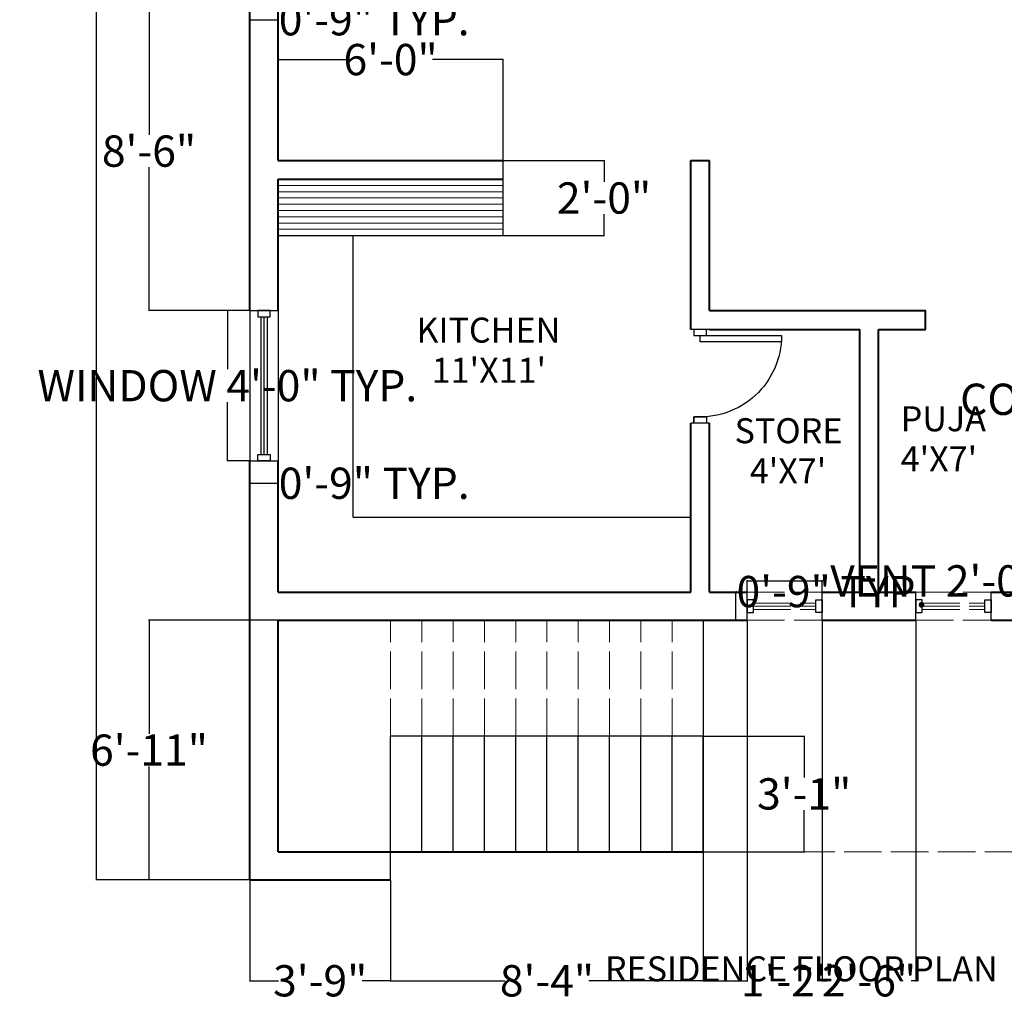
# Model space of a CAD drawing. Units: inches. Extents: x -413 to 212, y 1694 to 2633.
# Tile 2 of 5: x -413 to -98, y 1966 to 2279. Entities that reach past the tile are written whole.
import ezdxf

# ---------------------------------------------------------------- set-up
doc = ezdxf.new("R2010")
doc.units = ezdxf.units.IN
doc.header["$MEASUREMENT"] = 0
doc.linetypes.add('ACAD_ISO02W100', pattern=[15, 12, -3])
for name, color, linetype, lineweight in [('A-ANNO-DIMS', 5, 'Continuous', 18), ('A-ANNO-TEXT', 251, 'Continuous', 35), ('A-AREA-IDEN', 251, 'Continuous', 25), ('A-FLOR-FIXT', 1, 'Continuous', 25), ('A-FLOR-FIXT-PATT', 1, 'Continuous', 13), ('A-FLOR-OVHD', 20, 'ACAD_ISO02W100', 18), ('A-FLOR-STRS-OVHD', 3, 'ACAD_ISO02W100', 18), ('A-GLAZ-OVHD', 2, 'ACAD_ISO02W100', 18), ('A-GLAZ-VENT', 2, 'Continuous', 25), ('door', 4, 'Continuous', 25), ('stair case', 3, 'Continuous', 25), ('wall', 20, 'Continuous', 40), ('window', 6, 'Continuous', 25)]:
    doc.layers.add(name, color=color, linetype=linetype, lineweight=lineweight)
doc.styles.get("Standard").update_dxf_attribs({"font": 'arial.ttf'})
doc.dimstyles.get("Standard").update_dxf_attribs({"dimtxt": 10, "dimasz": 0.18, "dimexe": 0.18, "dimexo": 0.0625, "dimgap": 0.09, "dimtad": 0, "dimtih": 1, "dimtoh": 1, "dimdec": 1, "dimzin": 0, "dimdsep": 46, "dimlunit": 3, "dimtxsty": 'Standard', "dimblk": 'ARCHTICK', "dimcen": 0.09, "dimadec": 0, "dimazin": 0, "dimtfac": 1, "dimtdec": 1, "dimtofl": 0, "dimtmove": 0, "dimatfit": 3, "dimfxl": 1, "dimtolj": 1, "dimtzin": 0, "dimarcsym": 0})

# ---------------------------------------------------------------- blocks, each defined once
blk = doc.blocks.new('_ArchTick')
at = {"color": 0, "linetype": 'ByBlock', "const_width": 0.15}
blk.add_lwpolyline([(-0.5, -0.5), (0.5, 0.5)], dxfattribs=at)
blk = doc.blocks.new('*D2')
at = {"layer": 'A-ANNO-DIMS', "color": 0, "lineweight": -2, "transparency": 16777216}
for p, q in [((-339.04, 2585.48), (-388.23, 2585.48)), ((-388.05, 2585.48), (-388.05, 2300.18)), ((-388.05, 2004.48), (-388.05, 2289.79)), ((-339.04, 2004.48), (-388.23, 2004.48))]:
    blk.add_line(p, q, dxfattribs=at)
at = {"layer": 'Defpoints', "color": 0, "transparency": 16777216}
for p in [(-388.05, 2585.48), (-338.98, 2585.48), (-338.98, 2004.48)]:
    blk.add_point(p, dxfattribs=at)
at = {"layer": 'A-ANNO-DIMS', "color": 0, "lineweight": -2, "transparency": 16777216, "xscale": 0.18, "yscale": 0.18, "zscale": 0.18}
for p, rotation in [((-388.05, 2585.48), 90), ((-388.05, 2004.48), 270)]:
    blk.add_blockref('_ArchTick', p, dxfattribs=dict(at, rotation=rotation))
at = {"layer": 'A-ANNO-DIMS', "color": 0, "transparency": 16777216, "insert": (-388.05, 2294.98), "char_height": 10, "attachment_point": 5}
blk.add_mtext('\\A1;48\'-5.0"', dxfattribs=at)
blk = doc.blocks.new('WINDOW-48IN')
for p, q in [((0, 0), (0, 9)), ((0, 9), (48, 9)), ((48, 0), (48, 9)), ((2, 5.5), (46, 5.5)), ((2, 4.5), (46, 4.5)), ((2, 3.5), (46, 3.5)), ((0, 0), (48, 0))]:
    blk.add_line(p, q)
for points in [[(0, 2.5), (2, 2.5), (2, 6.5), (0, 6.5)], [(48, 2.5), (46, 2.5), (46, 6.5), (48, 6.5)]]:
    blk.add_lwpolyline(points, close=True)
blk = doc.blocks.new('VENT-JAMBS-24IN')
for p, q in [((0, 0), (0, 9)), ((24, 0), (24, 9))]:
    blk.add_line(p, q)
for points in [[(0, 2.5), (2, 2.5), (2, 6.5), (0, 6.5)], [(24, 2.5), (22, 2.5), (22, 6.5), (24, 6.5)]]:
    blk.add_lwpolyline(points, close=True)
blk = doc.blocks.new('VENT-PANEL-24IN')
for p, q in [((0, 9), (24, 9)), ((2, 5.5), (22, 5.5)), ((2, 4.5), (22, 4.5)), ((2, 3.5), (22, 3.5)), ((0, 0), (24, 0))]:
    blk.add_line(p, q)
blk = doc.blocks.new('DOOR-SWING-30IN')
for points in [[(0, 0), (0, 26), (-2, 26), (-2, 0)], [(-28, -2), (-26, -2), (-26, 2), (-28, 2)], [(2, -2), (0, -2), (0, 2), (2, 2)]]:
    blk.add_lwpolyline(points, close=True)
blk.add_arc((0, 0), 26, 90, 184.4117)
blk = doc.blocks.new('*D27')
at = {"layer": 'A-ANNO-DIMS', "color": 0, "lineweight": -2, "transparency": 16777216}
for p, q in [((-339.04, 2186.48), (-346.36, 2186.48)), ((-346.18, 2186.48), (-346.18, 2167.75)), ((-346.18, 2138.48), (-346.18, 2157.22)), ((-339.04, 2138.48), (-346.36, 2138.48))]:
    blk.add_line(p, q, dxfattribs=at)
at = {"layer": 'Defpoints', "color": 0, "transparency": 16777216}
for p in [(-338.98, 2186.48), (-346.18, 2138.48), (-338.98, 2138.48)]:
    blk.add_point(p, dxfattribs=at)
at = {"layer": 'A-ANNO-DIMS', "color": 0, "lineweight": -2, "transparency": 16777216, "xscale": 0.18, "yscale": 0.18, "zscale": 0.18}
for p, rotation in [((-346.18, 2186.48), 90), ((-346.18, 2138.48), 270)]:
    blk.add_blockref('_ArchTick', p, dxfattribs=dict(at, rotation=rotation))
at = {"layer": 'A-ANNO-DIMS', "color": 0, "transparency": 16777216, "insert": (-346.18, 2162.48), "char_height": 10, "attachment_point": 5}
blk.add_mtext('\\A1;WINDOW 4\'-0" TYP.', dxfattribs=at)
blk = doc.blocks.new('*D28')
at = {"layer": 'A-ANNO-DIMS', "color": 0, "lineweight": -2, "transparency": 16777216}
for p, q in [((-338.98, 2138.42), (-338.98, 2131.1)), ((-329.98, 2138.42), (-329.98, 2131.1)), ((-338.98, 2131.28), (-329.98, 2131.28)), ((-329.98, 2131.28), (-329.8, 2131.28))]:
    blk.add_line(p, q, dxfattribs=at)
at = {"layer": 'Defpoints', "color": 0, "transparency": 16777216}
for p in [(-338.98, 2138.48), (-329.98, 2138.48), (-329.98, 2131.28)]:
    blk.add_point(p, dxfattribs=at)
at = {"layer": 'A-ANNO-DIMS', "color": 0, "lineweight": -2, "transparency": 16777216, "xscale": 0.18, "yscale": 0.18, "zscale": 0.18, "rotation": 180}
blk.add_blockref('_ArchTick', (-338.98, 2131.28), dxfattribs=at)
at = {"layer": 'A-ANNO-DIMS', "color": 0, "lineweight": -2, "transparency": 16777216, "xscale": 0.18, "yscale": 0.18, "zscale": 0.18}
blk.add_blockref('_ArchTick', (-329.98, 2131.28), dxfattribs=at)
at = {"layer": 'A-ANNO-DIMS', "color": 0, "transparency": 16777216, "insert": (-299.23, 2131.28), "char_height": 10, "attachment_point": 5}
blk.add_mtext('\\A1;0\'-9" TYP.', dxfattribs=at)
blk = doc.blocks.new('*D30')
at = {"layer": 'A-ANNO-DIMS', "color": 0, "lineweight": -2, "transparency": 16777216}
for p, q in [((-338.98, 2288.42), (-338.98, 2279.3)), ((-329.98, 2288.42), (-329.98, 2279.3)), ((-338.98, 2279.48), (-329.98, 2279.48)), ((-329.98, 2279.48), (-329.8, 2279.48))]:
    blk.add_line(p, q, dxfattribs=at)
at = {"layer": 'Defpoints', "color": 0, "transparency": 16777216}
for p in [(-338.98, 2288.48), (-329.98, 2288.48), (-329.98, 2279.48)]:
    blk.add_point(p, dxfattribs=at)
at = {"layer": 'A-ANNO-DIMS', "color": 0, "lineweight": -2, "transparency": 16777216, "xscale": 0.18, "yscale": 0.18, "zscale": 0.18, "rotation": 180}
blk.add_blockref('_ArchTick', (-338.98, 2279.48), dxfattribs=at)
at = {"layer": 'A-ANNO-DIMS', "color": 0, "lineweight": -2, "transparency": 16777216, "xscale": 0.18, "yscale": 0.18, "zscale": 0.18}
blk.add_blockref('_ArchTick', (-329.98, 2279.48), dxfattribs=at)
at = {"layer": 'A-ANNO-DIMS', "color": 0, "transparency": 16777216, "insert": (-299.23, 2279.48), "char_height": 10, "attachment_point": 5}
blk.add_mtext('\\A1;0\'-9" TYP.', dxfattribs=at)
blk = doc.blocks.new('*D31')
at = {"layer": 'A-ANNO-DIMS', "color": 0, "lineweight": -2, "transparency": 16777216}
for p, q in [((-179.98, 2096.55), (-179.98, 2100.26)), ((-179.98, 2100.08), (-155.98, 2100.08)), ((-155.98, 2096.55), (-155.98, 2100.26)), ((-155.98, 2100.08), (-155.8, 2100.08))]:
    blk.add_line(p, q, dxfattribs=at)
at = {"layer": 'Defpoints', "color": 0, "transparency": 16777216}
for p in [(-155.98, 2100.08), (-179.98, 2096.48), (-155.98, 2096.48)]:
    blk.add_point(p, dxfattribs=at)
at = {"layer": 'A-ANNO-DIMS', "color": 0, "lineweight": -2, "transparency": 16777216, "xscale": 0.18, "yscale": 0.18, "zscale": 0.18, "rotation": 180}
blk.add_blockref('_ArchTick', (-179.98, 2100.08), dxfattribs=at)
at = {"layer": 'A-ANNO-DIMS', "color": 0, "lineweight": -2, "transparency": 16777216, "xscale": 0.18, "yscale": 0.18, "zscale": 0.18}
blk.add_blockref('_ArchTick', (-155.98, 2100.08), dxfattribs=at)
at = {"layer": 'A-ANNO-DIMS', "color": 0, "transparency": 16777216, "insert": (-104.4, 2100.08), "char_height": 10, "attachment_point": 5}
blk.add_mtext('\\A1;VENT 2\'-0" TYP.', dxfattribs=at)
blk = doc.blocks.new('*D32')
at = {"layer": 'A-ANNO-DIMS', "color": 0, "lineweight": -2, "transparency": 16777216}
for p, q in [((-180.04, 2096.48), (-183.76, 2096.48)), ((-183.58, 2096.48), (-183.58, 2096.66)), ((-183.58, 2096.66), (-183.4, 2096.66)), ((-183.58, 2087.48), (-183.58, 2096.48)), ((-180.04, 2087.48), (-183.76, 2087.48))]:
    blk.add_line(p, q, dxfattribs=at)
at = {"layer": 'Defpoints', "color": 0, "transparency": 16777216}
for p in [(-183.58, 2096.48), (-179.98, 2096.48), (-179.98, 2087.48)]:
    blk.add_point(p, dxfattribs=at)
at = {"layer": 'A-ANNO-DIMS', "color": 0, "lineweight": -2, "transparency": 16777216, "xscale": 0.18, "yscale": 0.18, "zscale": 0.18}
for p, rotation in [((-183.58, 2096.48), 90), ((-183.58, 2087.48), 270)]:
    blk.add_blockref('_ArchTick', p, dxfattribs=dict(at, rotation=rotation))
at = {"layer": 'A-ANNO-DIMS', "color": 0, "transparency": 16777216, "insert": (-152.83, 2096.66), "char_height": 10, "attachment_point": 5}
blk.add_mtext('\\A1;0\'-9" TYP.', dxfattribs=at)
blk = doc.blocks.new('*D49')
at = {"layer": 'A-ANNO-DIMS', "color": 0, "lineweight": -2, "transparency": 16777216}
for p, q in [((-10.42, 2181.31), (-17.49, 2181.31)), ((-17.31, 2181.31), (-17.31, 2163.4)), ((-17.31, 2134.96), (-17.31, 2152.87)), ((-10.42, 2134.96), (-17.49, 2134.96))]:
    blk.add_line(p, q, dxfattribs=at)
at = {"layer": 'Defpoints', "color": 0, "transparency": 16777216}
for p in [(-10.36, 2181.31), (-17.31, 2134.96), (-10.36, 2134.96)]:
    blk.add_point(p, dxfattribs=at)
at = {"layer": 'A-ANNO-DIMS', "color": 0, "lineweight": -2, "transparency": 16777216, "xscale": 0.18, "yscale": 0.18, "zscale": 0.18}
for p, rotation in [((-17.31, 2181.31), 90), ((-17.31, 2134.96), 270)]:
    blk.add_blockref('_ArchTick', p, dxfattribs=dict(at, rotation=rotation))
at = {"layer": 'A-ANNO-DIMS', "color": 0, "transparency": 16777216, "insert": (-17.31, 2158.13), "char_height": 10, "attachment_point": 5}
blk.add_mtext('\\A1;COFFEE TABLE 3\'-10 1/2" TYP.', dxfattribs=at)
blk = doc.blocks.new('*D57')
at = {"layer": 'A-ANNO-DIMS', "color": 0, "lineweight": -2, "transparency": 16777216}
for p, q in [((-330.04, 2087.48), (-371.41, 2087.48)), ((-371.23, 2087.48), (-371.23, 2051.18)), ((-371.23, 2004.48), (-371.23, 2040.79)), ((-339.04, 2004.48), (-371.41, 2004.48))]:
    blk.add_line(p, q, dxfattribs=at)
at = {"layer": 'Defpoints', "color": 0, "transparency": 16777216}
for p in [(-371.23, 2087.48), (-329.98, 2087.48), (-338.98, 2004.48)]:
    blk.add_point(p, dxfattribs=at)
at = {"layer": 'A-ANNO-DIMS', "color": 0, "lineweight": -2, "transparency": 16777216, "xscale": 0.18, "yscale": 0.18, "zscale": 0.18}
for p, rotation in [((-371.23, 2087.48), 90), ((-371.23, 2004.48), 270)]:
    blk.add_blockref('_ArchTick', p, dxfattribs=dict(at, rotation=rotation))
at = {"layer": 'A-ANNO-DIMS', "color": 0, "transparency": 16777216, "insert": (-371.23, 2045.98), "char_height": 10, "attachment_point": 5}
blk.add_mtext('\\A1;6\'-11"', dxfattribs=at)
blk = doc.blocks.new('*D58')
at = {"layer": 'A-ANNO-DIMS', "color": 0, "lineweight": -2, "transparency": 16777216}
for p, q in [((-193.98, 2013.42), (-193.98, 1972.05)), ((-293.98, 2004.42), (-293.98, 1972.05)), ((-293.98, 1972.23), (-257.36, 1972.23)), ((-193.98, 1972.23), (-230.59, 1972.23))]:
    blk.add_line(p, q, dxfattribs=at)
at = {"layer": 'Defpoints', "color": 0, "transparency": 16777216}
for p in [(-193.98, 2013.48), (-293.98, 2004.48), (-193.98, 1972.23)]:
    blk.add_point(p, dxfattribs=at)
at = {"layer": 'A-ANNO-DIMS', "color": 0, "lineweight": -2, "transparency": 16777216, "xscale": 0.18, "yscale": 0.18, "zscale": 0.18, "rotation": 180}
blk.add_blockref('_ArchTick', (-293.98, 1972.23), dxfattribs=at)
at = {"layer": 'A-ANNO-DIMS', "color": 0, "lineweight": -2, "transparency": 16777216, "xscale": 0.18, "yscale": 0.18, "zscale": 0.18}
blk.add_blockref('_ArchTick', (-193.98, 1972.23), dxfattribs=at)
at = {"layer": 'A-ANNO-DIMS', "color": 0, "transparency": 16777216, "insert": (-243.98, 1972.23), "char_height": 10, "attachment_point": 5}
blk.add_mtext('\\A1;8\'-4"', dxfattribs=at)
blk = doc.blocks.new('*D59')
at = {"layer": 'A-ANNO-DIMS', "color": 0, "lineweight": -2, "transparency": 16777216}
for p, q in [((-338.98, 2004.42), (-338.98, 1972.05)), ((-293.98, 2004.42), (-293.98, 1972.05)), ((-338.98, 1972.23), (-329.85, 1972.23)), ((-293.98, 1972.23), (-303.1, 1972.23))]:
    blk.add_line(p, q, dxfattribs=at)
at = {"layer": 'Defpoints', "color": 0, "transparency": 16777216}
for p in [(-338.98, 2004.48), (-293.98, 2004.48), (-293.98, 1972.23)]:
    blk.add_point(p, dxfattribs=at)
at = {"layer": 'A-ANNO-DIMS', "color": 0, "lineweight": -2, "transparency": 16777216, "xscale": 0.18, "yscale": 0.18, "zscale": 0.18, "rotation": 180}
blk.add_blockref('_ArchTick', (-338.98, 1972.23), dxfattribs=at)
at = {"layer": 'A-ANNO-DIMS', "color": 0, "lineweight": -2, "transparency": 16777216, "xscale": 0.18, "yscale": 0.18, "zscale": 0.18}
blk.add_blockref('_ArchTick', (-293.98, 1972.23), dxfattribs=at)
at = {"layer": 'A-ANNO-DIMS', "color": 0, "transparency": 16777216, "insert": (-316.48, 1972.23), "char_height": 10, "attachment_point": 5}
blk.add_mtext('\\A1;3\'-9"', dxfattribs=at)
blk = doc.blocks.new('*D70')
at = {"layer": 'A-ANNO-DIMS', "color": 0, "lineweight": -2, "transparency": 16777216}
for p, q in [((-339.04, 2288.48), (-371.41, 2288.48)), ((-371.23, 2288.48), (-371.23, 2242.68)), ((-371.23, 2186.48), (-371.23, 2232.29)), ((-339.04, 2186.48), (-371.41, 2186.48))]:
    blk.add_line(p, q, dxfattribs=at)
at = {"layer": 'Defpoints', "color": 0, "transparency": 16777216}
for p in [(-338.98, 2288.48), (-371.23, 2186.48), (-338.98, 2186.48)]:
    blk.add_point(p, dxfattribs=at)
at = {"layer": 'A-ANNO-DIMS', "color": 0, "lineweight": -2, "transparency": 16777216, "xscale": 0.18, "yscale": 0.18, "zscale": 0.18}
for p, rotation in [((-371.23, 2288.48), 90), ((-371.23, 2186.48), 270)]:
    blk.add_blockref('_ArchTick', p, dxfattribs=dict(at, rotation=rotation))
at = {"layer": 'A-ANNO-DIMS', "color": 0, "transparency": 16777216, "insert": (-371.23, 2237.48), "char_height": 10, "attachment_point": 5}
blk.add_mtext('\\A1;8\'-6"', dxfattribs=at)
blk = doc.blocks.new('*D76')
at = {"layer": 'A-ANNO-DIMS', "color": 0, "lineweight": -2, "transparency": 16777216}
for p, q in [((-193.98, 2087.42), (-193.98, 1972.05)), ((-179.98, 2087.42), (-179.98, 1972.05)), ((-193.98, 1972.23), (-179.98, 1972.23)), ((-179.98, 1972.23), (-179.8, 1972.23))]:
    blk.add_line(p, q, dxfattribs=at)
at = {"layer": 'Defpoints', "color": 0, "transparency": 16777216}
for p in [(-193.98, 2087.48), (-179.98, 2087.48), (-179.98, 1972.23)]:
    blk.add_point(p, dxfattribs=at)
at = {"layer": 'A-ANNO-DIMS', "color": 0, "lineweight": -2, "transparency": 16777216, "xscale": 0.18, "yscale": 0.18, "zscale": 0.18, "rotation": 180}
blk.add_blockref('_ArchTick', (-193.98, 1972.23), dxfattribs=at)
at = {"layer": 'A-ANNO-DIMS', "color": 0, "lineweight": -2, "transparency": 16777216, "xscale": 0.18, "yscale": 0.18, "zscale": 0.18}
blk.add_blockref('_ArchTick', (-179.98, 1972.23), dxfattribs=at)
at = {"layer": 'A-ANNO-DIMS', "color": 0, "transparency": 16777216, "insert": (-166.89, 1972.23), "char_height": 10, "attachment_point": 5}
blk.add_mtext('\\A1;1\'-2"', dxfattribs=at)
blk = doc.blocks.new('*D77')
at = {"layer": 'A-ANNO-DIMS', "color": 0, "lineweight": -2, "transparency": 16777216}
for p, q in [((-155.98, 2087.42), (-155.98, 1972.05)), ((-125.98, 2087.42), (-125.98, 1972.05)), ((-155.98, 1972.23), (-154.44, 1972.23)), ((-125.98, 1972.23), (-127.51, 1972.23))]:
    blk.add_line(p, q, dxfattribs=at)
at = {"layer": 'Defpoints', "color": 0, "transparency": 16777216}
for p in [(-155.98, 2087.48), (-125.98, 2087.48), (-125.98, 1972.23)]:
    blk.add_point(p, dxfattribs=at)
at = {"layer": 'A-ANNO-DIMS', "color": 0, "lineweight": -2, "transparency": 16777216, "xscale": 0.18, "yscale": 0.18, "zscale": 0.18, "rotation": 180}
blk.add_blockref('_ArchTick', (-155.98, 1972.23), dxfattribs=at)
at = {"layer": 'A-ANNO-DIMS', "color": 0, "lineweight": -2, "transparency": 16777216, "xscale": 0.18, "yscale": 0.18, "zscale": 0.18}
blk.add_blockref('_ArchTick', (-125.98, 1972.23), dxfattribs=at)
at = {"layer": 'A-ANNO-DIMS', "color": 0, "transparency": 16777216, "insert": (-140.98, 1972.23), "char_height": 10, "attachment_point": 5}
blk.add_mtext('\\A1;2\'-6"', dxfattribs=at)
blk = doc.blocks.new('*D78')
at = {"layer": 'A-ANNO-DIMS', "color": 0, "lineweight": -2, "transparency": 16777216}
for p, q in [((-329.98, 2234.55), (-329.98, 2266.91)), ((-257.98, 2234.55), (-257.98, 2266.91)), ((-329.98, 2266.73), (-307.38, 2266.73)), ((-257.98, 2266.73), (-280.57, 2266.73))]:
    blk.add_line(p, q, dxfattribs=at)
at = {"layer": 'Defpoints', "color": 0, "transparency": 16777216}
for p in [(-257.98, 2266.73), (-329.98, 2234.48), (-257.98, 2234.48)]:
    blk.add_point(p, dxfattribs=at)
at = {"layer": 'A-ANNO-DIMS', "color": 0, "lineweight": -2, "transparency": 16777216, "xscale": 0.18, "yscale": 0.18, "zscale": 0.18, "rotation": 180}
blk.add_blockref('_ArchTick', (-329.98, 2266.73), dxfattribs=at)
at = {"layer": 'A-ANNO-DIMS', "color": 0, "lineweight": -2, "transparency": 16777216, "xscale": 0.18, "yscale": 0.18, "zscale": 0.18}
blk.add_blockref('_ArchTick', (-257.98, 2266.73), dxfattribs=at)
at = {"layer": 'A-ANNO-DIMS', "color": 0, "transparency": 16777216, "insert": (-293.98, 2266.73), "char_height": 10, "attachment_point": 5}
blk.add_mtext('\\A1;6\'-0"', dxfattribs=at)
blk = doc.blocks.new('*D79')
at = {"layer": 'A-ANNO-DIMS', "color": 0, "lineweight": -2, "transparency": 16777216}
for p, q in [((-257.91, 2234.48), (-225.55, 2234.48)), ((-225.73, 2234.48), (-225.73, 2227.68)), ((-225.73, 2210.48), (-225.73, 2217.29)), ((-257.91, 2210.48), (-225.55, 2210.48))]:
    blk.add_line(p, q, dxfattribs=at)
at = {"layer": 'Defpoints', "color": 0, "transparency": 16777216}
for p in [(-257.98, 2234.48), (-257.98, 2210.48), (-225.73, 2210.48)]:
    blk.add_point(p, dxfattribs=at)
at = {"layer": 'A-ANNO-DIMS', "color": 0, "lineweight": -2, "transparency": 16777216, "xscale": 0.18, "yscale": 0.18, "zscale": 0.18}
for p, rotation in [((-225.73, 2234.48), 90), ((-225.73, 2210.48), 270)]:
    blk.add_blockref('_ArchTick', p, dxfattribs=dict(at, rotation=rotation))
at = {"layer": 'A-ANNO-DIMS', "color": 0, "transparency": 16777216, "insert": (-225.73, 2222.48), "char_height": 10, "attachment_point": 5}
blk.add_mtext('\\A1;2\'-0"', dxfattribs=at)
blk = doc.blocks.new('*D80')
at = {"layer": 'A-ANNO-DIMS', "color": 0, "lineweight": -2, "transparency": 16777216}
for p, q in [((-193.91, 2050.48), (-161.55, 2050.48)), ((-161.73, 2050.48), (-161.73, 2037.18)), ((-161.73, 2013.48), (-161.73, 2026.79)), ((-193.91, 2013.48), (-161.55, 2013.48))]:
    blk.add_line(p, q, dxfattribs=at)
at = {"layer": 'Defpoints', "color": 0, "transparency": 16777216}
for p in [(-193.98, 2050.48), (-193.98, 2013.48), (-161.73, 2013.48)]:
    blk.add_point(p, dxfattribs=at)
at = {"layer": 'A-ANNO-DIMS', "color": 0, "lineweight": -2, "transparency": 16777216, "xscale": 0.18, "yscale": 0.18, "zscale": 0.18}
for p, rotation in [((-161.73, 2050.48), 90), ((-161.73, 2013.48), 270)]:
    blk.add_blockref('_ArchTick', p, dxfattribs=dict(at, rotation=rotation))
at = {"layer": 'A-ANNO-DIMS', "color": 0, "transparency": 16777216, "insert": (-161.73, 2031.98), "char_height": 10, "attachment_point": 5}
blk.add_mtext('\\A1;3\'-1"', dxfattribs=at)

msp = doc.modelspace()

# ---------------------------------------------------------------- hatches: boundary and pattern name
at = {"layer": 'A-FLOR-FIXT-PATT'}
h = msp.add_hatch(dxfattribs=at)
h.set_pattern_fill('ANSI31', color=256, scale=16.0035, angle=-45, style=0)
h.paths.add_polyline_path([(-329.98, 2210.48), (-257.98, 2210.48), (-257.98, 2228.48), (-329.98, 2228.48)])

# ---------------------------------------------------------------- linework, layer by layer
at = {"layer": 'A-FLOR-FIXT'}
for p, q in [((-257.98, 2210.48), (-257.98, 2234.48)), ((-329.98, 2210.48), (-257.98, 2210.48)), ((-305.98, 2120.48), (-305.98, 2210.48)), ((-305.98, 2120.48), (-197.98, 2120.48))]:
    msp.add_line(p, q, dxfattribs=at)
at = {"layer": 'A-FLOR-OVHD'}
msp.add_line((-193.98, 2013.48), (61.52, 2013.48), dxfattribs=at)
at = {"layer": 'A-FLOR-STRS-OVHD'}
for p, q in [((-293.98, 2050.48), (-293.98, 2087.48)), ((-283.98, 2050.48), (-283.98, 2087.48)), ((-273.98, 2050.48), (-273.98, 2087.48)), ((-263.98, 2050.48), (-263.98, 2087.48)), ((-253.98, 2050.48), (-253.98, 2087.48)), ((-243.98, 2050.48), (-243.98, 2087.48)), ((-233.98, 2050.48), (-233.98, 2087.48)), ((-223.98, 2050.48), (-223.98, 2087.48)), ((-213.98, 2050.48), (-213.98, 2087.48)), ((-203.98, 2050.48), (-203.98, 2087.48)), ((-193.98, 2050.48), (-193.98, 2087.48))]:
    msp.add_line(p, q, dxfattribs=at)
at = {"layer": 'door'}
for p, q in [((-191.98, 2180.48), (-197.98, 2180.48)), ((-196.98, 2180.48), (-196.98, 2178.48)), ((-191.98, 2150.48), (-197.98, 2150.48)), ((-196.98, 2152.56), (-196.98, 2150.48))]:
    msp.add_line(p, q, dxfattribs=at)
at = {"layer": 'stair case'}
for p, q in [((-293.98, 2004.48), (-293.98, 2050.48)), ((-193.98, 2050.48), (-293.98, 2050.48)), ((-283.98, 2013.48), (-283.98, 2050.48)), ((-273.98, 2013.48), (-273.98, 2050.48)), ((-263.98, 2013.48), (-263.98, 2050.48)), ((-253.98, 2013.48), (-253.98, 2050.48)), ((-243.98, 2013.48), (-243.98, 2050.48)), ((-233.98, 2013.48), (-233.98, 2050.48)), ((-223.98, 2013.48), (-223.98, 2050.48)), ((-213.98, 2013.48), (-213.98, 2050.48)), ((-203.98, 2013.48), (-203.98, 2050.48)), ((-193.98, 2013.48), (-193.98, 2050.48))]:
    msp.add_line(p, q, dxfattribs=at)
at = {"layer": 'wall'}
for p, q in [((-338.98, 2186.48), (-338.98, 2288.48)), ((-329.98, 2234.48), (-329.98, 2288.48)), ((-329.98, 2234.48), (-257.98, 2234.48)), ((-197.98, 2180.48), (-197.98, 2234.48)), ((-197.98, 2234.48), (-191.98, 2234.48)), ((-191.98, 2186.48), (-191.98, 2234.48)), ((-329.98, 2228.48), (-257.98, 2228.48)), ((-329.98, 2186.48), (-329.98, 2228.48)), ((-191.98, 2186.48), (-122.98, 2186.48)), ((-122.98, 2180.48), (-122.98, 2186.48)), ((-191.98, 2180.48), (-143.98, 2180.48)), ((-143.98, 2096.48), (-143.98, 2180.48)), ((-137.98, 2096.48), (-137.98, 2180.48)), ((-137.98, 2180.48), (-122.98, 2180.48)), ((-197.98, 2096.48), (-197.98, 2150.48)), ((-191.98, 2096.48), (-191.98, 2150.48)), ((-338.98, 2004.48), (-338.98, 2138.48)), ((-329.98, 2096.48), (-329.98, 2138.48)), ((-329.98, 2096.48), (-197.98, 2096.48)), ((-191.98, 2096.48), (-179.98, 2096.48)), ((-155.98, 2096.48), (-143.98, 2096.48)), ((-137.98, 2096.48), (-125.98, 2096.48)), ((-101.98, 2096.48), (-89.98, 2096.48)), ((-329.98, 2013.48), (-329.98, 2087.48)), ((-329.98, 2087.48), (-179.98, 2087.48)), ((-155.98, 2087.48), (-125.98, 2087.48)), ((-101.98, 2087.48), (-77.98, 2087.48)), ((-329.98, 2013.48), (-193.98, 2013.48)), ((-338.98, 2004.48), (-293.98, 2004.48)), ((-293.98, 2004.48), (-293.98, 2004.48))]:
    msp.add_line(p, q, dxfattribs=at)

# ---------------------------------------------------------------- block references
at = {"layer": 'A-GLAZ-OVHD'}
for p in [(-179.98, 2087.48), (-125.98, 2087.48)]:
    msp.add_blockref('VENT-PANEL-24IN', p, dxfattribs=at)
at = {"layer": 'A-GLAZ-VENT'}
for p in [(-179.98, 2087.48), (-125.98, 2087.48)]:
    msp.add_blockref('VENT-JAMBS-24IN', p, dxfattribs=at)
at = {"layer": 'door', "extrusion": (0, 0, -1), "zscale": -1, "rotation": 89.99999999999795}
msp.add_blockref('DOOR-SWING-30IN', (194.98, 2178.48), dxfattribs=at)
at = {"layer": 'window', "rotation": 270.0000000000044}
msp.add_blockref('WINDOW-48IN', (-338.98, 2186.48), dxfattribs=at)

# ---------------------------------------------------------------- texts
at = {"layer": 'A-ANNO-TEXT'}
msp.add_text('RESIDENCE FLOOR PLAN ', height=8, dxfattribs=at).set_placement((-225.45, 1972.05))
at = {"layer": 'A-AREA-IDEN'}
for s, p in [('KITCHEN ', (-285.72, 2176.25)), ("  11'X11'", (-285.72, 2163.4)), ('PUJA ', (-130.87, 2147.9)), ('STORE ', (-184, 2144.08)), ("4'X7'", (-130.87, 2135.05)), ("  4'X7'", (-184, 2131.23))]:
    msp.add_text(s, height=8, dxfattribs=at).set_placement(p)

# ---------------------------------------------------------------- dimensions: what is measured, and where the dimension line sits
at = {"layer": 'A-ANNO-DIMS'}
for base, p1, p2, angle, override, picture, middle in [((-388.05, 2585.48), (-338.98, 2004.48), (-338.98, 2585.48), 90, {"dimclrd": 0, "dimclre": 0, "dimclrt": 0}, '*D2', (-388.05, 2294.98)), ((-371.23, 2186.48), (-338.98, 2288.48), (-338.98, 2186.48), 90, {"dimdec": 1, "dimlfac": 1, "dimrnd": 0, "dimzin": 1, "dimdsep": 46, "dimlunit": 4, "dimfrac": 2}, '*D70', (-371.23, 2237.48)), ((-225.73, 2210.48), (-257.98, 2234.48), (-257.98, 2210.48), 270, {"dimdec": 1, "dimlfac": 1, "dimrnd": 0, "dimzin": 1, "dimdsep": 46, "dimlunit": 4, "dimfrac": 2}, '*D79', (-225.73, 2222.48)), ((-371.23, 2087.48), (-338.98, 2004.48), (-329.98, 2087.48), 90, {"dimdec": 1, "dimlfac": 1, "dimrnd": 0, "dimzin": 1, "dimdsep": 46, "dimlunit": 4, "dimfrac": 2}, '*D57', (-371.23, 2045.98)), ((-161.73, 2013.48), (-193.98, 2050.48), (-193.98, 2013.48), 270, {"dimdec": 1, "dimlfac": 1, "dimrnd": 0, "dimzin": 1, "dimdsep": 46, "dimlunit": 4, "dimfrac": 2}, '*D80', (-161.73, 2031.98))]:
    dim = msp.add_linear_dim(base=base, p1=p1, p2=p2, angle=angle, dimstyle='Standard', override=override, dxfattribs=at)
    dim.commit()
    dim.dimension.update_dxf_attribs({"geometry": picture, "text_midpoint": middle})
for base, p1, p2, text, picture, middle in [((-329.98, 2279.48), (-338.98, 2288.48), (-329.98, 2288.48), '<> TYP.', '*D30', (-299.23, 2279.48)), ((-155.98, 2100.08), (-179.98, 2096.48), (-155.98, 2096.48), 'VENT <> TYP.', '*D31', (-104.4, 2100.08))]:
    dim = msp.add_linear_dim(base=base, p1=p1, p2=p2, text=text, dimstyle='Standard', override={"dimdec": 1, "dimlfac": 1, "dimrnd": 0, "dimzin": 1, "dimdsep": 46, "dimlunit": 4, "dimfrac": 2}, dxfattribs=at)
    dim.commit()
    dim.dimension.update_dxf_attribs({"geometry": picture, "text_midpoint": middle})
for base, p1, p2, picture, middle in [((-257.98, 2266.73), (-329.98, 2234.48), (-257.98, 2234.48), '*D78', (-293.98, 2266.73)), ((-179.98, 1972.23), (-193.98, 2087.48), (-179.98, 2087.48), '*D76', (-166.89, 1972.23)), ((-125.98, 1972.23), (-155.98, 2087.48), (-125.98, 2087.48), '*D77', (-140.98, 1972.23)), ((-193.98, 1972.23), (-293.98, 2004.48), (-193.98, 2013.48), '*D58', (-243.98, 1972.23)), ((-293.98, 1972.23), (-338.98, 2004.48), (-293.98, 2004.48), '*D59', (-316.48, 1972.23))]:
    dim = msp.add_linear_dim(base=base, p1=p1, p2=p2, dimstyle='Standard', override={"dimdec": 1, "dimlfac": 1, "dimrnd": 0, "dimzin": 1, "dimdsep": 46, "dimlunit": 4, "dimfrac": 2}, dxfattribs=at)
    dim.commit()
    dim.dimension.update_dxf_attribs({"geometry": picture, "text_midpoint": middle})
for base, p1, p2, angle, text, picture, middle in [((-17.312, 2134.9599), (-10.3595, 2181.3098), (-10.3595, 2134.9599), 270, 'COFFEE TABLE <> TYP.', '*D49', (-17.312, 2158.1349)), ((-346.18, 2138.48), (-338.98, 2186.48), (-338.98, 2138.48), 270, 'WINDOW <> TYP.', '*D27', (-346.18, 2162.48)), ((-329.98, 2131.28), (-338.98, 2138.48), (-329.98, 2138.48), 0, '<> TYP.', '*D28', (-299.23, 2131.28)), ((-183.58, 2096.48), (-179.98, 2087.48), (-179.98, 2096.48), 90, '<> TYP.', '*D32', (-152.83, 2096.66))]:
    dim = msp.add_linear_dim(base=base, p1=p1, p2=p2, angle=angle, text=text, dimstyle='Standard', override={"dimdec": 1, "dimlfac": 1, "dimrnd": 0, "dimzin": 1, "dimdsep": 46, "dimlunit": 4, "dimfrac": 2}, dxfattribs=at)
    dim.commit()
    dim.dimension.update_dxf_attribs({"geometry": picture, "text_midpoint": middle})

doc.saveas('drawing.dxf')
